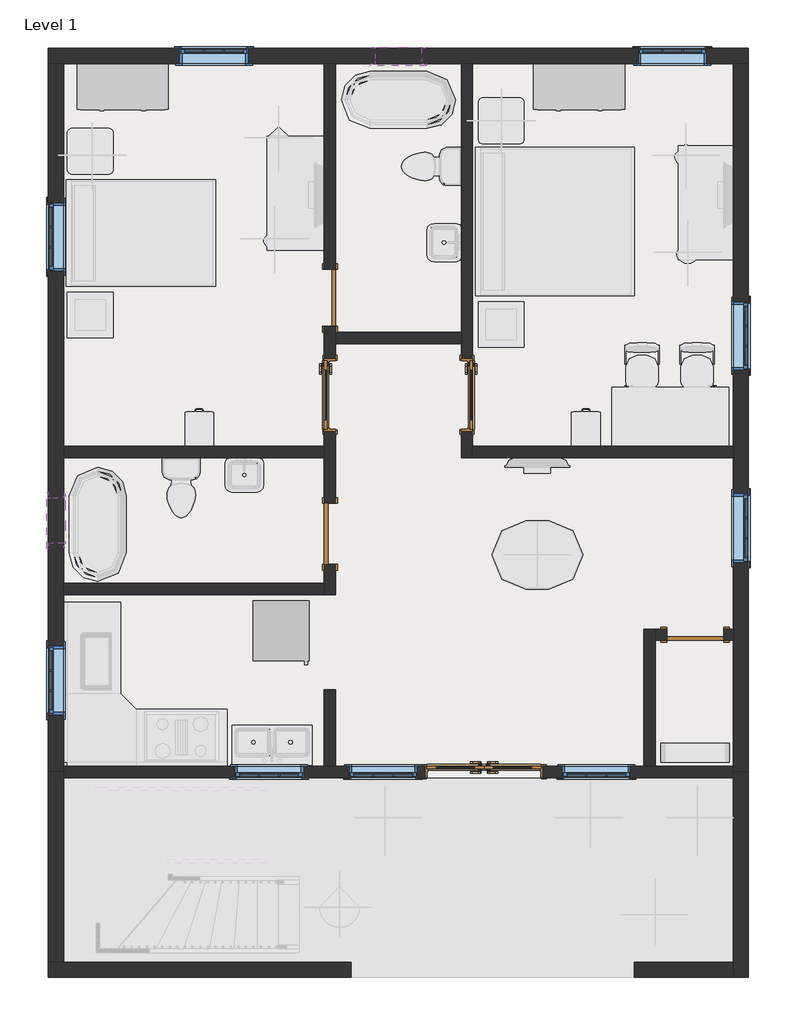
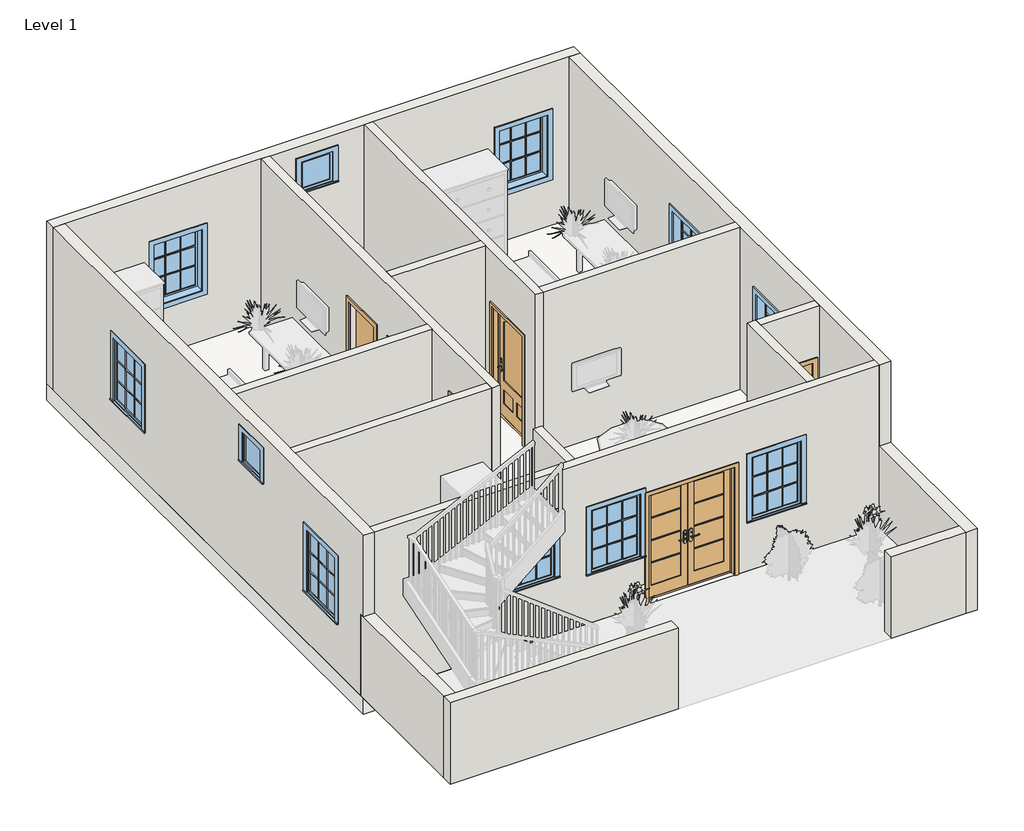
# One storey, part 1 of 3: 17 walls, 11 windows, 6 doors, 1 slab.
"""IFC4 building model written with IfcOpenShell, lengths in millimetres."""

from ifc_helpers import new_model, si_unit, frame, origin, origin_with_axes, place, context, project, spatial, polyline, outline, extrude, faceted_brep, transform, mapped, element, save
from components import door_808aeb8e, door_5d363d20, door_94998e6c, door_059fdd7e, door_bb092f7c, window_29c06734, window_5c190c7e, window_e41d21a6

model = new_model("IFC4")

# Units and contexts
model_context = context("Model", 3, world=origin())
ifc_project = project(units=[si_unit("LENGTHUNIT", "METRE", prefix="MILLI")], contexts=[model_context])

# Site, building, storey
site = spatial("IfcSite", under=ifc_project)
building = spatial("IfcBuilding", under=site)
storey = spatial("IfcBuildingStorey", under=building, Name="Level 1", Elevation=0.0)

# Doors
placement = place(None, origin())
door_shape = door_808aeb8e(model_context)
element("IfcDoor", 1, ObjectType="36\" x 80\"", at=placement, inside=storey, context=model_context, shape_type="MappedRepresentation", body=[
    mapped(door_shape, transform((-7676.9823372, 9599.5174997, 0.0), x_axis=(0.0, 1.0, 0.0), y_axis=(-1.0, 0.0, 0.0), z_axis=(0.0, 0.0, 1.0))),
])
door_2_shape = door_5d363d20(model_context)
element("IfcDoor", 2, ObjectType="36\" x 80\"", at=placement, inside=storey, context=model_context, shape_type="MappedRepresentation", body=[
    mapped(door_2_shape, transform((-5841.8323372, 9599.5174997, 0.0), x_axis=(0.0, 1.0, 0.0), y_axis=(-1.0, 0.0, 0.0), z_axis=(0.0, 0.0, 1.0))),
])
door_3_shape = door_94998e6c(model_context)
element("IfcDoor", 3, ObjectType="Door-Exterior-Double-Full Glass-Wood_Clad : 60\" x 80\"", at=placement, inside=storey, context=model_context, shape_type="MappedRepresentation", body=[
    mapped(door_3_shape, transform((-5616.4073372, 4573.4924997, 0.0), x_axis=(1.0, 0.0, 0.0), y_axis=(0.0, 1.0, 0.0), z_axis=(0.0, 0.0, 1.0))),
])
door_4_shape = door_059fdd7e(model_context)
element("IfcDoor", 4, ObjectType="Single-Flush : 30\" x 80\"", at=placement, inside=storey, context=model_context, shape_type="MappedRepresentation", body=[
    mapped(door_4_shape, transform((-2797.0073372, 6399.1174997, 0.0), x_axis=(-1.0, 0.0, 0.0), y_axis=(0.0, -1.0, 0.0), z_axis=(0.0, 0.0, 1.0))),
])
element("IfcDoor", 5, ObjectType="Single-Flush : 30\" x 80\"", at=placement, inside=storey, context=model_context, shape_type="MappedRepresentation", body=[
    mapped(door_4_shape, transform((-7673.8073372, 10894.9174997, 0.0), x_axis=(0.0, -1.0, 0.0), y_axis=(1.0, 0.0, 0.0), z_axis=(0.0, 0.0, 1.0))),
])
door_5_shape = door_bb092f7c(model_context)
element("IfcDoor", 6, ObjectType="Single-Flush : 32\" x 84\"", at=placement, inside=storey, context=model_context, shape_type="MappedRepresentation", body=[
    mapped(door_5_shape, transform((-7673.8073372, 7745.3174997, 0.0), x_axis=(0.0, -1.0, 0.0), y_axis=(1.0, 0.0, 0.0), z_axis=(0.0, 0.0, 1.0))),
])

# Slab
element("IfcSlab", 7, ObjectType="Generic - 12\"", at=placement, inside=storey, context=model_context, shape_type="SweptSolid", body=[
    extrude(outline(polyline([(-2085.8073372, 14222.3174997), (-2085.8073372, 4494.1174997), (-11433.0073372, 4494.1174997), (-11433.0073372, 14222.3174997), (-2085.8073372, 14222.3174997)])), frame((0.0, 0.0, -304.8), z_axis=(0.0, 0.0, 1.0), x_axis=(1.0, 0.0, 0.0)), (0.0, 0.0, 1.0), 304.8),
])

# Walls
element("IfcWall", 8, ObjectType="Generic - 5'", at=placement, inside=storey, context=model_context, shape_type="SweptSolid", body=[
    extrude(outline(polyline([(-3609.8073372, 2030.3174997), (-2289.0073372, 2030.3174997), (-2289.0073372, 1827.1174997), (-3609.8073372, 1827.1174997), (-3609.8073372, 2030.3174997)])), origin_with_axes(), (0.0, 0.0, 1.0), 1524.0),
])
element("IfcWall", 9, ObjectType="Generic - 5'", at=placement, inside=storey, context=model_context, shape_type="Brep", body=[
    faceted_brep([(-11229.8073372, 2030.3174997, 0.0), (-11229.8073372, 4494.1174997, 0.0), (-11229.8073372, 4570.3174997, 0.0), (-11229.8073372, 4570.3174997, 1524.0), (-11229.8073372, 2030.3174997, 1524.0), (-11433.0073372, 2030.3174997, 0.0), (-11433.0073372, 2030.3174997, 1524.0), (-11433.0073372, 4570.3174997, 1524.0), (-11433.0073372, 4570.3174997, 0.0)], [[[0, 1, 2, 3, 4]], [[5, 6, 7, 8]], [[2, 1, 0, 5, 8]], [[3, 2, 8, 7]], [[4, 3, 7, 6]], [[0, 4, 6, 5]]]),
])
element("IfcWall", 10, ObjectType="Generic - 5'", at=placement, inside=storey, context=model_context, shape_type="Brep", body=[
    faceted_brep([(-2289.0073372, 4570.3174997, 0.0), (-2289.0073372, 4494.1174997, 0.0), (-2289.0073372, 2030.3174997, 0.0), (-2289.0073372, 1827.1174997, 0.0), (-2289.0073372, 1827.1174997, 1524.0), (-2289.0073372, 2030.3174997, 1524.0), (-2289.0073372, 4570.3174997, 1524.0), (-2085.8073372, 4570.3174997, 0.0), (-2085.8073372, 4570.3174997, 1524.0), (-2085.8073372, 1827.1174997, 1524.0), (-2085.8073372, 1827.1174997, 0.0)], [[[0, 1, 2, 3, 4, 5, 6]], [[7, 8, 9, 10]], [[3, 2, 1, 0, 7, 10]], [[6, 5, 4, 9, 8]], [[0, 6, 8, 7]], [[4, 3, 10, 9]]]),
])
element("IfcWall", 11, ObjectType="Generic - 5'", at=placement, inside=storey, context=model_context, shape_type="Brep", body=[
    faceted_brep([(-7394.4073372, 2030.3174997, 0.0), (-11229.8073372, 2030.3174997, 0.0), (-11433.0073372, 2030.3174997, 0.0), (-11433.0073372, 2030.3174997, 1524.0), (-11229.8073372, 2030.3174997, 1524.0), (-7394.4073372, 2030.3174997, 1524.0), (-7394.4073372, 1827.1174997, 0.0), (-7394.4073372, 1827.1174997, 1524.0), (-11433.0073372, 1827.1174997, 1524.0), (-11433.0073372, 1827.1174997, 0.0)], [[[0, 1, 2, 3, 4, 5]], [[6, 7, 8, 9]], [[2, 1, 0, 6, 9]], [[5, 4, 3, 8, 7]], [[0, 5, 7, 6]], [[3, 2, 9, 8]]]),
])
element("IfcWall", 12, ObjectType="Generic - 8\"", at=placement, inside=storey, context=model_context, shape_type="Brep", body=[
    faceted_brep([(-11433.0073372, 14019.1174997, 0.0), (-11229.8073372, 14019.1174997, 0.0), (-7750.0073372, 14019.1174997, 0.0), (-7597.6073372, 14019.1174997, 0.0), (-5921.2073372, 14019.1174997, 0.0), (-5768.8073372, 14019.1174997, 0.0), (-2289.0073372, 14019.1174997, 0.0), (-2085.8073372, 14019.1174997, 0.0), (-2085.8073372, 14019.1174997, 3048.0), (-2289.0073372, 14019.1174997, 3048.0), (-5768.8073372, 14019.1174997, 3048.0), (-5921.2073372, 14019.1174997, 3048.0), (-7597.6073372, 14019.1174997, 3048.0), (-7750.0073372, 14019.1174997, 3048.0), (-11229.8073372, 14019.1174997, 3048.0), (-11433.0073372, 14019.1174997, 3048.0), (-8766.0073372, 14019.1174997, 2133.6), (-8766.0073372, 14019.1174997, 914.4), (-9680.4073372, 14019.1174997, 914.4), (-9680.4073372, 14019.1174997, 2133.6), (-2644.6073372, 14019.1174997, 2133.6), (-2644.6073372, 14019.1174997, 914.4), (-3559.0073372, 14019.1174997, 914.4), (-3559.0073372, 14019.1174997, 2133.6), (-7064.2073372, 14019.1174997, 2768.6), (-6454.6073372, 14019.1174997, 2768.6), (-6454.6073372, 14019.1174997, 2159.0), (-7064.2073372, 14019.1174997, 2159.0), (-11433.0073372, 14222.3174997, 0.0), (-11433.0073372, 14222.3174997, 3048.0), (-2085.8073372, 14222.3174997, 3048.0), (-2085.8073372, 14222.3174997, 0.0), (-8766.0073372, 14222.3174997, 2133.6), (-9680.4073372, 14222.3174997, 2133.6), (-9680.4073372, 14222.3174997, 914.4), (-8766.0073372, 14222.3174997, 914.4), (-2644.6073372, 14222.3174997, 2133.6), (-3559.0073372, 14222.3174997, 2133.6), (-3559.0073372, 14222.3174997, 914.4), (-2644.6073372, 14222.3174997, 914.4), (-7064.2073372, 14222.3174997, 2768.6), (-7064.2073372, 14222.3174997, 2159.0), (-6454.6073372, 14222.3174997, 2159.0), (-6454.6073372, 14222.3174997, 2768.6)], [[[0, 1, 2, 3, 4, 5, 6, 7, 8, 9, 10, 11, 12, 13, 14, 15], [16, 17, 18, 19], [20, 21, 22, 23], [24, 25, 26, 27]], [[28, 29, 30, 31], [32, 33, 34, 35], [36, 37, 38, 39], [40, 41, 42, 43]], [[7, 6, 5, 4, 3, 2, 1, 0, 28, 31]], [[8, 7, 31, 30]], [[0, 15, 29, 28]], [[17, 16, 32, 35]], [[18, 17, 35, 34]], [[19, 18, 34, 33]], [[16, 19, 33, 32]], [[21, 20, 36, 39]], [[22, 21, 39, 38]], [[23, 22, 38, 37]], [[20, 23, 37, 36]], [[41, 40, 24, 27]], [[42, 41, 27, 26]], [[43, 42, 26, 25]], [[40, 43, 25, 24]], [[15, 14, 13, 12, 11, 10, 9, 8, 30, 29]]]),
])
element("IfcWall", 13, ObjectType="Generic - 8\"", at=placement, inside=storey, context=model_context, shape_type="Brep", body=[
    faceted_brep([(-2289.0073372, 14019.1174997, 0.0), (-2289.0073372, 8913.7174997, 0.0), (-2289.0073372, 8761.3174997, 0.0), (-2289.0073372, 6475.3174997, 0.0), (-2289.0073372, 6322.9174997, 0.0), (-2289.0073372, 4646.5174997, 0.0), (-2289.0073372, 4570.3174997, 0.0), (-2289.0073372, 4570.3174997, 1524.0), (-2289.0073372, 4494.1174997, 1524.0), (-2289.0073372, 4494.1174997, 3048.0), (-2289.0073372, 4646.5174997, 3048.0), (-2289.0073372, 6322.9174997, 3048.0), (-2289.0073372, 6475.3174997, 3048.0), (-2289.0073372, 8761.3174997, 3048.0), (-2289.0073372, 8913.7174997, 3048.0), (-2289.0073372, 14019.1174997, 3048.0), (-2289.0073372, 7364.3174997, 2133.6), (-2289.0073372, 7364.3174997, 914.4), (-2289.0073372, 8278.7174997, 914.4), (-2289.0073372, 8278.7174997, 2133.6), (-2289.0073372, 9929.7174997, 2133.6), (-2289.0073372, 9929.7174997, 914.4), (-2289.0073372, 10844.1174997, 914.4), (-2289.0073372, 10844.1174997, 2133.6), (-2085.8073372, 14019.1174997, 0.0), (-2085.8073372, 14019.1174997, 3048.0), (-2085.8073372, 4494.1174997, 3048.0), (-2085.8073372, 4494.1174997, 1524.0), (-2085.8073372, 4570.3174997, 1524.0), (-2085.8073372, 4570.3174997, 0.0), (-2085.8073372, 7364.3174997, 2133.6), (-2085.8073372, 8278.7174997, 2133.6), (-2085.8073372, 8278.7174997, 914.4), (-2085.8073372, 7364.3174997, 914.4), (-2085.8073372, 9929.7174997, 2133.6), (-2085.8073372, 10844.1174997, 2133.6), (-2085.8073372, 10844.1174997, 914.4), (-2085.8073372, 9929.7174997, 914.4)], [[[0, 1, 2, 3, 4, 5, 6, 7, 8, 9, 10, 11, 12, 13, 14, 15], [16, 17, 18, 19], [20, 21, 22, 23]], [[24, 25, 26, 27, 28, 29], [30, 31, 32, 33], [34, 35, 36, 37]], [[6, 5, 4, 3, 2, 1, 0, 24, 29]], [[0, 15, 25, 24]], [[17, 16, 30, 33]], [[18, 17, 33, 32]], [[19, 18, 32, 31]], [[16, 19, 31, 30]], [[21, 20, 34, 37]], [[22, 21, 37, 36]], [[23, 22, 36, 35]], [[20, 23, 35, 34]], [[7, 6, 29, 28]], [[27, 8, 7, 28]], [[9, 8, 27, 26]], [[15, 14, 13, 12, 11, 10, 9, 26, 25]]]),
])
element("IfcWall", 14, ObjectType="Generic - 8\"", at=placement, inside=storey, context=model_context, shape_type="Brep", body=[
    faceted_brep([(-11229.8073372, 4570.3174997, 0.0), (-11229.8073372, 4646.5174997, 0.0), (-11229.8073372, 6932.5174997, 0.0), (-11229.8073372, 7084.9174997, 0.0), (-11229.8073372, 8761.3174997, 0.0), (-11229.8073372, 8913.7174997, 0.0), (-11229.8073372, 14019.1174997, 0.0), (-11229.8073372, 14019.1174997, 3048.0), (-11229.8073372, 8913.7174997, 3048.0), (-11229.8073372, 8761.3174997, 3048.0), (-11229.8073372, 7084.9174997, 3048.0), (-11229.8073372, 6932.5174997, 3048.0), (-11229.8073372, 4646.5174997, 3048.0), (-11229.8073372, 4494.1174997, 3048.0), (-11229.8073372, 4494.1174997, 1524.0), (-11229.8073372, 4570.3174997, 1524.0), (-11229.8073372, 12164.9174997, 2133.6), (-11229.8073372, 12164.9174997, 914.4), (-11229.8073372, 11250.5174997, 914.4), (-11229.8073372, 11250.5174997, 2133.6), (-11229.8073372, 6246.7174997, 2133.6), (-11229.8073372, 6246.7174997, 914.4), (-11229.8073372, 5332.3174997, 914.4), (-11229.8073372, 5332.3174997, 2133.6), (-11229.8073372, 8227.9174997, 2768.6), (-11229.8073372, 8227.9174997, 2159.0), (-11229.8073372, 7618.3174997, 2159.0), (-11229.8073372, 7618.3174997, 2768.6), (-11433.0073372, 4570.3174997, 0.0), (-11433.0073372, 4570.3174997, 1524.0), (-11433.0073372, 4494.1174997, 1524.0), (-11433.0073372, 4494.1174997, 3048.0), (-11433.0073372, 14019.1174997, 3048.0), (-11433.0073372, 14019.1174997, 0.0), (-11433.0073372, 12164.9174997, 2133.6), (-11433.0073372, 11250.5174997, 2133.6), (-11433.0073372, 11250.5174997, 914.4), (-11433.0073372, 12164.9174997, 914.4), (-11433.0073372, 6246.7174997, 2133.6), (-11433.0073372, 5332.3174997, 2133.6), (-11433.0073372, 5332.3174997, 914.4), (-11433.0073372, 6246.7174997, 914.4), (-11433.0073372, 8227.9174997, 2768.6), (-11433.0073372, 7618.3174997, 2768.6), (-11433.0073372, 7618.3174997, 2159.0), (-11433.0073372, 8227.9174997, 2159.0)], [[[0, 1, 2, 3, 4, 5, 6, 7, 8, 9, 10, 11, 12, 13, 14, 15], [16, 17, 18, 19], [20, 21, 22, 23], [24, 25, 26, 27]], [[28, 29, 30, 31, 32, 33], [34, 35, 36, 37], [38, 39, 40, 41], [42, 43, 44, 45]], [[6, 5, 4, 3, 2, 1, 0, 28, 33]], [[7, 6, 33, 32]], [[17, 16, 34, 37]], [[18, 17, 37, 36]], [[19, 18, 36, 35]], [[16, 19, 35, 34]], [[21, 20, 38, 41]], [[22, 21, 41, 40]], [[23, 22, 40, 39]], [[20, 23, 39, 38]], [[25, 24, 42, 45]], [[26, 25, 45, 44]], [[27, 26, 44, 43]], [[24, 27, 43, 42]], [[0, 15, 29, 28]], [[14, 30, 29, 15]], [[14, 13, 31, 30]], [[13, 12, 11, 10, 9, 8, 7, 32, 31]]]),
])
element("IfcWall", 15, ObjectType="INNER 6\"", at=placement, inside=storey, context=model_context, shape_type="Brep", body=[
    faceted_brep([(-7750.0073372, 10513.9174997, 2032.0), (-7750.0073372, 10513.9174997, 0.0), (-7750.0073372, 10082.1174997, 0.0), (-7750.0073372, 10082.1174997, 2057.4), (-7750.0073372, 9116.9174997, 2057.4), (-7750.0073372, 9116.9174997, 0.0), (-7750.0073372, 8913.7174997, 0.0), (-7750.0073372, 8761.3174997, 0.0), (-7750.0073372, 8151.7174997, 0.0), (-7750.0073372, 8151.7174997, 2133.6), (-7750.0073372, 7338.9174997, 2133.6), (-7750.0073372, 7338.9174997, 0.0), (-7750.0073372, 7084.9174997, 0.0), (-7750.0073372, 6932.5174997, 0.0), (-7750.0073372, 6932.5174997, 3048.0), (-7750.0073372, 7084.9174997, 3048.0), (-7750.0073372, 8761.3174997, 3048.0), (-7750.0073372, 8913.7174997, 3048.0), (-7750.0073372, 14019.1174997, 3048.0), (-7750.0073372, 14019.1174997, 0.0), (-7750.0073372, 11275.9174997, 0.0), (-7750.0073372, 11275.9174997, 2032.0), (-7597.6073372, 10082.1174997, 0.0), (-7597.6073372, 10285.3174997, 0.0), (-7597.6073372, 10437.7174997, 0.0), (-7597.6073372, 10513.9174997, 0.0), (-7597.6073372, 10513.9174997, 2032.0), (-7597.6073372, 11275.9174997, 2032.0), (-7597.6073372, 11275.9174997, 0.0), (-7597.6073372, 14019.1174997, 0.0), (-7597.6073372, 14019.1174997, 3048.0), (-7597.6073372, 10437.7174997, 3048.0), (-7597.6073372, 10285.3174997, 3048.0), (-7597.6073372, 6932.5174997, 3048.0), (-7597.6073372, 6932.5174997, 0.0), (-7597.6073372, 7338.9174997, 0.0), (-7597.6073372, 7338.9174997, 2133.6), (-7597.6073372, 8151.7174997, 2133.6), (-7597.6073372, 8151.7174997, 0.0), (-7597.6073372, 9116.9174997, 0.0), (-7597.6073372, 9116.9174997, 2057.4), (-7597.6073372, 10082.1174997, 2057.4)], [[[0, 1, 2, 3, 4, 5, 6, 7, 8, 9, 10, 11, 12, 13, 14, 15, 16, 17, 18, 19, 20, 21]], [[22, 23, 24, 25, 26, 27, 28, 29, 30, 31, 32, 33, 34, 35, 36, 37, 38, 39, 40, 41]], [[11, 35, 34, 13, 12]], [[38, 8, 7, 6, 5, 39]], [[20, 19, 29, 28]], [[2, 1, 25, 24, 23, 22]], [[19, 18, 30, 29]], [[36, 35, 11, 10]], [[37, 36, 10, 9]], [[38, 37, 9, 8]], [[41, 3, 2, 22]], [[3, 41, 40, 4]], [[4, 40, 39, 5]], [[14, 13, 34, 33]], [[26, 25, 1, 0]], [[27, 26, 0, 21]], [[28, 27, 21, 20]], [[18, 17, 16, 15, 14, 33, 32, 31, 30]]]),
])
element("IfcWall", 16, ObjectType="INNER 6\"", at=placement, inside=storey, context=model_context, shape_type="SweptSolid", body=[
    extrude(outline(polyline([(-11229.8073372, 8913.7174997), (-7750.0073372, 8913.7174997), (-7750.0073372, 8761.3174997), (-11229.8073372, 8761.3174997), (-11229.8073372, 8913.7174997)])), origin_with_axes(), (0.0, 0.0, 1.0), 3048.0),
])
element("IfcWall", 17, ObjectType="INNER 6\"", at=placement, inside=storey, context=model_context, shape_type="Brep", body=[
    faceted_brep([(-5921.2073372, 14019.1174997, 3048.0), (-5921.2073372, 14019.1174997, 0.0), (-5921.2073372, 10437.7174997, 0.0), (-5921.2073372, 10285.3174997, 0.0), (-5921.2073372, 10082.1174997, 0.0), (-5921.2073372, 10082.1174997, 2057.4), (-5921.2073372, 9116.9174997, 2057.4), (-5921.2073372, 9116.9174997, 0.0), (-5921.2073372, 8761.3174997, 0.0), (-5921.2073372, 8761.3174997, 3048.0), (-5921.2073372, 10285.3174997, 3048.0), (-5921.2073372, 10437.7174997, 3048.0), (-5768.8073372, 14019.1174997, 0.0), (-5768.8073372, 14019.1174997, 3048.0), (-5768.8073372, 8913.7174997, 3048.0), (-5768.8073372, 8761.3174997, 3048.0), (-5768.8073372, 8761.3174997, 0.0), (-5768.8073372, 8913.7174997, 0.0), (-5768.8073372, 9116.9174997, 0.0), (-5768.8073372, 9116.9174997, 2057.4), (-5768.8073372, 10082.1174997, 2057.4), (-5768.8073372, 10082.1174997, 0.0)], [[[0, 1, 2, 3, 4, 5, 6, 7, 8, 9, 10, 11]], [[12, 13, 14, 15, 16, 17, 18, 19, 20, 21]], [[1, 12, 21, 4, 3, 2]], [[16, 8, 7, 18, 17]], [[1, 0, 13, 12]], [[9, 8, 16, 15]], [[20, 5, 4, 21]], [[5, 20, 19, 6]], [[6, 19, 18, 7]], [[0, 11, 10, 9, 15, 14, 13]]]),
])
element("IfcWall", 18, ObjectType="INNER 6\"", at=placement, inside=storey, context=model_context, shape_type="SweptSolid", body=[
    extrude(outline(polyline([(-7597.6073372, 10437.7174997), (-5921.2073372, 10437.7174997), (-5921.2073372, 10285.3174997), (-7597.6073372, 10285.3174997), (-7597.6073372, 10437.7174997)])), origin_with_axes(), (0.0, 0.0, 1.0), 3048.0),
])
element("IfcWall", 19, ObjectType="INNER 6\"", at=placement, inside=storey, context=model_context, shape_type="SweptSolid", body=[
    extrude(outline(polyline([(-2289.0073372, 8761.3174997), (-5768.8073372, 8761.3174997), (-5768.8073372, 8913.7174997), (-2289.0073372, 8913.7174997), (-2289.0073372, 8761.3174997)])), origin_with_axes(), (0.0, 0.0, 1.0), 3048.0),
])
element("IfcWall", 20, ObjectType="INNER 6\"", at=placement, inside=storey, context=model_context, shape_type="SweptSolid", body=[
    extrude(outline(polyline([(-7750.0073372, 6932.5174997), (-11229.8073372, 6932.5174997), (-11229.8073372, 7084.9174997), (-7750.0073372, 7084.9174997), (-7750.0073372, 6932.5174997)])), origin_with_axes(), (0.0, 0.0, 1.0), 3048.0),
])
element("IfcWall", 21, ObjectType="INNER 6\"", at=placement, inside=storey, context=model_context, shape_type="Brep", body=[
    faceted_brep([(-2289.0073372, 4494.1174997, 0.0), (-2289.0073372, 4494.1174997, 1524.0), (-2289.0073372, 4494.1174997, 3048.0), (-11229.8073372, 4494.1174997, 3048.0), (-11229.8073372, 4494.1174997, 1524.0), (-11229.8073372, 4494.1174997, 0.0), (-6403.8073372, 4494.1174997, 0.0), (-6403.8073372, 4494.1174997, 2057.4), (-4829.0073372, 4494.1174997, 2057.4), (-4829.0073372, 4494.1174997, 0.0), (-8943.8073372, 4494.1174997, 2286.0), (-8029.4073372, 4494.1174997, 2286.0), (-8029.4073372, 4494.1174997, 1066.8), (-8943.8073372, 4494.1174997, 1066.8), (-7419.8073372, 4494.1174997, 2133.6), (-6505.4073372, 4494.1174997, 2133.6), (-6505.4073372, 4494.1174997, 914.4), (-7419.8073372, 4494.1174997, 914.4), (-4575.0073372, 4494.1174997, 2133.6), (-3660.6073372, 4494.1174997, 2133.6), (-3660.6073372, 4494.1174997, 914.4), (-4575.0073372, 4494.1174997, 914.4), (-2289.0073372, 4646.5174997, 3048.0), (-2289.0073372, 4646.5174997, 0.0), (-3330.4073372, 4646.5174997, 0.0), (-3482.8073372, 4646.5174997, 0.0), (-4829.0073372, 4646.5174997, 0.0), (-4829.0073372, 4646.5174997, 2057.4), (-6403.8073372, 4646.5174997, 2057.4), (-6403.8073372, 4646.5174997, 0.0), (-7597.6073372, 4646.5174997, 0.0), (-7750.0073372, 4646.5174997, 0.0), (-11229.8073372, 4646.5174997, 0.0), (-11229.8073372, 4646.5174997, 3048.0), (-7750.0073372, 4646.5174997, 3048.0), (-7597.6073372, 4646.5174997, 3048.0), (-3482.8073372, 4646.5174997, 3048.0), (-3330.4073372, 4646.5174997, 3048.0), (-8943.8073372, 4646.5174997, 2286.0), (-8943.8073372, 4646.5174997, 1066.8), (-8029.4073372, 4646.5174997, 1066.8), (-8029.4073372, 4646.5174997, 2286.0), (-7419.8073372, 4646.5174997, 2133.6), (-7419.8073372, 4646.5174997, 914.4), (-6505.4073372, 4646.5174997, 914.4), (-6505.4073372, 4646.5174997, 2133.6), (-4575.0073372, 4646.5174997, 2133.6), (-4575.0073372, 4646.5174997, 914.4), (-3660.6073372, 4646.5174997, 914.4), (-3660.6073372, 4646.5174997, 2133.6), (-2289.0073372, 4570.3174997, 0.0), (-11229.8073372, 4570.3174997, 0.0)], [[[0, 1, 2, 3, 4, 5, 6, 7, 8, 9], [10, 11, 12, 13], [14, 15, 16, 17], [18, 19, 20, 21]], [[22, 23, 24, 25, 26, 27, 28, 29, 30, 31, 32, 33, 34, 35, 36, 37], [38, 39, 40, 41], [42, 43, 44, 45], [46, 47, 48, 49]], [[23, 50, 0, 9, 26, 25, 24]], [[5, 51, 32, 31, 30, 29, 6]], [[8, 27, 26, 9]], [[27, 8, 7, 28]], [[28, 7, 6, 29]], [[39, 38, 10, 13]], [[40, 39, 13, 12]], [[41, 40, 12, 11]], [[38, 41, 11, 10]], [[43, 42, 14, 17]], [[44, 43, 17, 16]], [[45, 44, 16, 15]], [[42, 45, 15, 14]], [[47, 46, 18, 21]], [[48, 47, 21, 20]], [[49, 48, 20, 19]], [[46, 49, 19, 18]], [[0, 50, 23, 22, 2, 1]], [[32, 51, 5, 4, 3, 33]], [[3, 2, 22, 37, 36, 35, 34, 33]]]),
])
element("IfcWall", 22, ObjectType="INNER 6\"", at=placement, inside=storey, context=model_context, shape_type="Brep", body=[
    faceted_brep([(-3330.4073372, 4646.5174997, 0.0), (-3330.4073372, 6322.9174997, 0.0), (-3330.4073372, 6475.3174997, 0.0), (-3330.4073372, 6475.3174997, 3048.0), (-3330.4073372, 6322.9174997, 3048.0), (-3330.4073372, 4646.5174997, 3048.0), (-3482.8073372, 4646.5174997, 0.0), (-3482.8073372, 4646.5174997, 3048.0), (-3482.8073372, 6475.3174997, 3048.0), (-3482.8073372, 6475.3174997, 0.0)], [[[0, 1, 2, 3, 4, 5]], [[6, 7, 8, 9]], [[2, 1, 0, 6, 9]], [[0, 5, 7, 6]], [[3, 2, 9, 8]], [[5, 4, 3, 8, 7]]]),
])
element("IfcWall", 23, ObjectType="INNER 6\"", at=placement, inside=storey, context=model_context, shape_type="SweptSolid", body=[
    extrude(outline(polyline([(0.0, -3330.4073372), (0.0, -3178.0073372), (2032.0, -3178.0073372), (2032.0, -2416.0073372), (0.0, -2416.0073372), (0.0, -2289.0073372), (3048.0, -2289.0073372), (3048.0, -3330.4073372), (0.0, -3330.4073372)])), frame((0.0, 6322.9174997, 0.0), z_axis=(0.0, 1.0, 0.0), x_axis=(0.0, 0.0, 1.0)), (0.0, 0.0, 1.0), 152.4),
])
element("IfcWall", 24, ObjectType="INNER 6\"", at=placement, inside=storey, context=model_context, shape_type="SweptSolid", body=[
    extrude(outline(polyline([(-7750.0073372, 4646.5174997), (-7750.0073372, 5662.5174997), (-7597.6073372, 5662.5174997), (-7597.6073372, 4646.5174997), (-7750.0073372, 4646.5174997)])), origin_with_axes(), (0.0, 0.0, 1.0), 3048.0),
])

# Windows
window_shape = window_29c06734(model_context)
element("IfcWindow", 25, ObjectType="Casement 3x3 with Trim : 36\" x 48\"", at=placement, inside=storey, context=model_context, shape_type="MappedRepresentation", body=[
    mapped(window_shape, transform((-9223.2073372, 14120.7174997, 0.0), x_axis=(1.0, 0.0, 0.0), y_axis=(0.0, 1.0, 0.0), z_axis=(0.0, 0.0, 1.0))),
])
element("IfcWindow", 26, ObjectType="Casement 3x3 with Trim : 36\" x 48\"", at=placement, inside=storey, context=model_context, shape_type="MappedRepresentation", body=[
    mapped(window_shape, transform((-11331.4073372, 11707.7174997, 0.0), x_axis=(0.0, 1.0, 0.0), y_axis=(-1.0, 0.0, 0.0), z_axis=(0.0, 0.0, 1.0))),
])
element("IfcWindow", 27, ObjectType="Casement 3x3 with Trim : 36\" x 48\"", at=placement, inside=storey, context=model_context, shape_type="MappedRepresentation", body=[
    mapped(window_shape, transform((-11331.4073372, 5789.5174997, 0.0), x_axis=(0.0, 1.0, 0.0), y_axis=(-1.0, 0.0, 0.0), z_axis=(0.0, 0.0, 1.0))),
])
element("IfcWindow", 28, ObjectType="Casement 3x3 with Trim : 36\" x 48\"", at=placement, inside=storey, context=model_context, shape_type="MappedRepresentation", body=[
    mapped(window_shape, transform((-2187.4073372, 7821.5174997, 0.0), x_axis=(0.0, -1.0, 0.0), y_axis=(1.0, 0.0, 0.0), z_axis=(0.0, 0.0, 1.0))),
])
element("IfcWindow", 29, ObjectType="Casement 3x3 with Trim : 36\" x 48\"", at=placement, inside=storey, context=model_context, shape_type="MappedRepresentation", body=[
    mapped(window_shape, transform((-2187.4073372, 10386.9174997, 0.0), x_axis=(0.0, -1.0, 0.0), y_axis=(1.0, 0.0, 0.0), z_axis=(0.0, 0.0, 1.0))),
])
element("IfcWindow", 30, ObjectType="Casement 3x3 with Trim : 36\" x 48\"", at=placement, inside=storey, context=model_context, shape_type="MappedRepresentation", body=[
    mapped(window_shape, transform((-3101.8073372, 14120.7174997, 0.0), x_axis=(1.0, 0.0, 0.0), y_axis=(0.0, 1.0, 0.0), z_axis=(0.0, 0.0, 1.0))),
])
window_2_shape = window_5c190c7e(model_context)
element("IfcWindow", 31, ObjectType="Casement 3x3 with Trim : 36\" x 48\"", at=placement, inside=storey, context=model_context, shape_type="MappedRepresentation", body=[
    mapped(window_2_shape, transform((-8486.6073372, 4570.3174997, 152.4), x_axis=(-1.0, 0.0, 0.0), y_axis=(0.0, -1.0, 0.0), z_axis=(0.0, 0.0, 1.0))),
])
element("IfcWindow", 32, ObjectType="Casement 3x3 with Trim : 36\" x 48\"", at=placement, inside=storey, context=model_context, shape_type="MappedRepresentation", body=[
    mapped(window_2_shape, transform((-6962.6073372, 4570.3174997, 0.0), x_axis=(-1.0, 0.0, 0.0), y_axis=(0.0, -1.0, 0.0), z_axis=(0.0, 0.0, 1.0))),
])
element("IfcWindow", 33, ObjectType="Casement 3x3 with Trim : 36\" x 48\"", at=placement, inside=storey, context=model_context, shape_type="MappedRepresentation", body=[
    mapped(window_2_shape, transform((-4117.8073372, 4570.3174997, 0.0), x_axis=(-1.0, 0.0, 0.0), y_axis=(0.0, -1.0, 0.0), z_axis=(0.0, 0.0, 1.0))),
])
window_3_shape = window_e41d21a6(model_context)
element("IfcWindow", 34, ObjectType="Transom with Trim : 24\" x 24\"", at=placement, inside=storey, context=model_context, shape_type="MappedRepresentation", body=[
    mapped(window_3_shape, transform((-6797.5073372, 14120.7174997, 0.0), x_axis=(-1.0, 0.0, 0.0), y_axis=(0.0, -1.0, 0.0), z_axis=(0.0, 0.0, 1.0))),
])
element("IfcWindow", 35, ObjectType="Transom with Trim : 24\" x 24\"", at=placement, inside=storey, context=model_context, shape_type="MappedRepresentation", body=[
    mapped(window_3_shape, transform((-11331.4073372, 7961.2174997, 0.0), x_axis=(0.0, 1.0, 0.0), y_axis=(-1.0, 0.0, 0.0), z_axis=(0.0, 0.0, 1.0))),
])

save(model, "model.ifc")

# Revit data of these elements
# Type "36\" x 80\""
#   Type Mark = "8"
#   Assembly Code = "B2030100"
#   Analytic Construction = "French door, wood frame with single glass"
#   Threshold Offset [instance default] = 0' - 0 1/2"
#   Thickness = 0' - 1 3/8"
#   Thermal Resistance (R) = 1.0696 (h·ft²·°F)/BTU
#   Swing Angle [instance default] = 90.00°
#   Stiles = 0' - 4 3/4"
#   Rough Width = 3' - 2"
#   Rough Height = 6' - 9"
#   Radius = 1' - 8.05625"
#   Lock Rail = 0' - 7 1/8"
#   Height = 6' - 8"
#   Width = 3' - 0"
#   Heat Transfer Coefficient (U) = 0.9350 BTU/(h·ft²·°F)
#   Door Offset [instance default] = 0' - 0"
#   Bottom Rail = 0' - 9 1/2"
#   Threshold [instance default] = yes
#   Function = 1
#   Exterior Trim [instance default] = yes
#   Trim Material = Cherry
#   Threshold Material = Cherry
#   Panel Material = Cherry
#   Glazing = Glass
#   Frame Material = Cherry
#   Door Handle Material = Aluminum
#   Visual Light Transmittance = 0
#   Solar Heat Gain Coefficient = 0
#   Wall Closure = (empty or 0)
#   Construction Type = (empty or 0)
# Type "Door-Exterior-Double-Full Glass-Wood_Clad : 60\" x 80\""
#   Type Mark = "9"
#   Assembly Code = "B2030100"
#   Analytic Construction = "French door, wood frame with double glass"
#   Top Rail = 0' - 4 11/16"
#   Threshold Offset [instance default] = 0' - 0 1/2"
#   Thickness = 0' - 1 3/8"
#   Thermal Resistance (R) = 1.9158 (h·ft²·°F)/BTU
#   Swing Angle [instance default] = 90.00°
#   Stiles = 0' - 4 3/4"
#   Rough Width = 5' - 2"
#   Rough Height = 6' - 9"
#   Panel Width = 2' - 6"
#   Door Offset [instance default] = 0' - 0"
#   Height = 6' - 8"
#   Width = 5' - 0"
#   Heat Transfer Coefficient (U) = 0.5220 BTU/(h·ft²·°F)
#   Bottom Rail = 0' - 9 1/8"
#   Exterior Trim [instance default] = yes
#   Threshold [instance default] = yes
#   Show Grill [instance default] = yes
#   Function = 1
#   Trim Material = Cherry
#   Threshold Material = Cherry
#   Panel Material = Cherry
#   Glazing = Glass
#   Frame Material = Cherry
#   Door Handle Material = Aluminum
#   Visual Light Transmittance = 0
#   Solar Heat Gain Coefficient = 0
#   Wall Closure = (empty or 0)
#   Construction Type = (empty or 0)
# Type "Single-Flush : 30\" x 80\""
#   Type Mark = "5"
#   Construction Type Id = "MDOOR"
#   Assembly Code = "C1020"
#   Analytic Construction = "Metal"
#   Thickness = 0' - 2"
#   Heat Transfer Coefficient (U) = 0.651978 BTU/(h·ft²·°F)
#   Height = 6' - 8"
#   Trim Projection Ext = 0' - 1"
#   Trim Projection Int = 0' - 1"
#   Trim Width = 0' - 3"
#   Width = 2' - 6"
#   Define Thermal Properties by = 1
#   Door Material = Door - Panel
#   Frame Material = Door - Frame
#   Visual Light Transmittance = 0
#   Solar Heat Gain Coefficient = 0
#   Function = (empty or 0)
#   Wall Closure = (empty or 0)
# Type "Single-Flush : 32\" x 84\""
#   Type Mark = "3"
#   Construction Type Id = "MDOOR"
#   Assembly Code = "C1020"
#   Analytic Construction = "Metal"
#   Thickness = 0' - 2"
#   Heat Transfer Coefficient (U) = 0.651978 BTU/(h·ft²·°F)
#   Height = 7' - 0"
#   Trim Projection Ext = 0' - 1"
#   Trim Projection Int = 0' - 1"
#   Trim Width = 0' - 3"
#   Width = 2' - 8"
#   Define Thermal Properties by = 1
#   Door Material = Door - Panel
#   Frame Material = Door - Frame
#   Visual Light Transmittance = 0
#   Solar Heat Gain Coefficient = 0
#   Function = (empty or 0)
#   Wall Closure = (empty or 0)
# Type "Generic - 12\""
#   Assembly Code = "B1010"
#   Function = 0
#   Layers, outside or top first: 1' - 0" no material (function 1)
# Type "Generic - 5'"
#   Assembly Code = "B2010"
#   Layers, outside or top first: 0' - 8" "Birch" (function 1)
# Type "Generic - 8\""
#   Assembly Code = "B2010"
#   Layers, outside or top first: 0' - 8" "Brick, Common" (function 1)
# Type "INNER 6\""
#   Assembly Code = "B2010"
#   Layers, outside or top first: 0' - 6" "Brick, Common" (function 1)
# Type "Casement 3x3 with Trim : 36\" x 48\""
#   Type Mark = "10"
#   Construction Type Id = "GSP4R"
#   Assembly Code = "B2020100"
#   Analytic Construction = "1/8 in Pilkington single glazing"
#   Visual Light Transmittance = 0.9
#   Solar Heat Gain Coefficient = 0.78
#   Heat Transfer Coefficient (U) = 0.6496 BTU/(h·ft²·°F)
#   Height = 4' - 0"
#   Default Sill Height = 3' - 0"
#   Trim Projection - Ext. = 0' - 0 1/2"
#   Trim Projection - Int. = 0' - 0 3/4"
#   Trim Width - Exterior = 0' - 3 1/2"
#   Trim Width - Interior = 0' - 3 1/2"
#   Width = 3' - 0"
#   Window Inset = 0' - 0 3/4"
#   Define Thermal Properties by = 1
#   Glass Pane Material = Glass
#   Sash Material = Sash
#   Trim Exterior Material = Trim
#   Trim Interior Material = Trim
#   Wall Closure = (empty or 0)
# Type "Transom with Trim : 24\" x 24\""
#   Type Mark = "13"
#   Construction Type Id = "GSP4R"
#   Assembly Code = "B2020100"
#   Analytic Construction = "1/8 in Pilkington single glazing"
#   Visual Light Transmittance = 0.9
#   Solar Heat Gain Coefficient = 0.78
#   Heat Transfer Coefficient (U) = 0.6496 BTU/(h·ft²·°F)
#   Height = 2' - 0"
#   Default Sill Height = 7' - 1"
#   Trim Projection - Ext. = 0' - 0 1/2"
#   Trim Projection - Int. = 0' - 0 3/4"
#   Trim Width - Exterior = 0' - 3 1/2"
#   Trim Width - Interior = 0' - 3 1/2"
#   Width = 2' - 0"
#   Window Inset = 0' - 0 3/4"
#   Define Thermal Properties by = 1
#   Glass Pane Material = Glass
#   Sash Material = Sash
#   Trim Exterior Material = Trim
#   Trim Interior Material = Trim
#   Wall Closure = (empty or 0)
# Elements 1, 2 (IfcDoor, "36\" x 80\"")
#   Threshold Offset = 0' - 0 1/2"
#   Swing Angle = 90.00°
#   Door Offset = 0' - 0"
#   Threshold = yes
#   Exterior Trim = yes
#   Phase Created = New Construction
#   Materials on its faces: "Cherry", "Aluminum", "Glass"
# Element 3 (IfcDoor, "Door-Exterior-Double-Full Glass-Wood_Clad : 60\" x 80\"")
#   Threshold Offset = 0' - 0 1/2"
#   Swing Angle = 90.00°
#   Door Offset = 0' - 0"
#   Threshold = yes
#   Show Grill = yes
#   Exterior Trim = yes
#   Phase Created = New Construction
#   Materials on its faces: "Cherry", "Aluminum", "Glass"
# Elements 4, 5 (IfcDoor, "Single-Flush : 30\" x 80\"")
#   Phase Created = New Construction
#   Materials on its faces: "Door - Frame", "Door - Panel"
# Element 6 (IfcDoor, "Single-Flush : 32\" x 84\"")
#   Phase Created = New Construction
#   Materials on its faces: "Door - Frame", "Door - Panel"
# Element 7 (IfcSlab, "Generic - 12\"")
#   Height Offset From Level = 0' - 0"
#   Phase Created = New Construction
#   Materials on its faces: "Default Floor"
# Elements 8, 9, 10, 11 (IfcWall, "Generic - 5'")
#   Top Offset = 0' - 0"
#   Base Offset = 0' - 0"
#   Unconnected Height = 5' - 0"
#   wall height = 5' - 0"
#   Phase Created = New Construction
#   Base Constraint = Level 1
#   Materials on its faces: "Birch"
# Elements 12, 13, 14 (IfcWall, "Generic - 8\"")
#   Top Offset = 0' - 0"
#   Base Offset = 0' - 0"
#   Unconnected Height = 10' - 0"
#   wall height = 10' - 0"
#   Phase Created = New Construction
#   Base Constraint = Level 1
#   Materials on its faces: "Brick, Common"
# Elements 15, 16, 17, 18, 19, 20, 21, 22, 23, 24 (IfcWall, "INNER 6\"")
#   Top Offset = 0' - 0"
#   Base Offset = 0' - 0"
#   Unconnected Height = 10' - 0"
#   wall height = 10' - 0"
#   Phase Created = New Construction
#   Base Constraint = Level 1
#   Materials on its faces: "Brick, Common"
# Element 25 (IfcWindow, "Casement 3x3 with Trim : 36\" x 48\"")
#   Mark = "1"
#   Phase Created = New Construction
#   Materials on its faces: "Sash", "Glass", "Trim"
# Element 26 (IfcWindow, "Casement 3x3 with Trim : 36\" x 48\"")
#   Mark = "2"
#   Phase Created = New Construction
#   Materials on its faces: "Sash", "Glass", "Trim"
# Element 27 (IfcWindow, "Casement 3x3 with Trim : 36\" x 48\"")
#   Mark = "3"
#   Phase Created = New Construction
#   Materials on its faces: "Sash", "Glass", "Trim"
# Element 28 (IfcWindow, "Casement 3x3 with Trim : 36\" x 48\"")
#   Mark = "8"
#   Phase Created = New Construction
#   Materials on its faces: "Sash", "Glass", "Trim"
# Element 29 (IfcWindow, "Casement 3x3 with Trim : 36\" x 48\"")
#   Mark = "9"
#   Phase Created = New Construction
#   Materials on its faces: "Sash", "Glass", "Trim"
# Element 30 (IfcWindow, "Casement 3x3 with Trim : 36\" x 48\"")
#   Mark = "10"
#   Phase Created = New Construction
#   Materials on its faces: "Sash", "Glass", "Trim"
# Element 31 (IfcWindow, "Casement 3x3 with Trim : 36\" x 48\"")
#   Mark = "4"
#   Phase Created = New Construction
#   Materials on its faces: "Sash", "Glass", "Trim"
# Element 32 (IfcWindow, "Casement 3x3 with Trim : 36\" x 48\"")
#   Mark = "6"
#   Phase Created = New Construction
#   Materials on its faces: "Sash", "Glass", "Trim"
# Element 33 (IfcWindow, "Casement 3x3 with Trim : 36\" x 48\"")
#   Mark = "7"
#   Phase Created = New Construction
#   Materials on its faces: "Sash", "Glass", "Trim"
# Element 34 (IfcWindow, "Transom with Trim : 24\" x 24\"")
#   Mark = "11"
#   Phase Created = New Construction
#   Materials on its faces: "Sash", "Trim", "Glass"
# Element 35 (IfcWindow, "Transom with Trim : 24\" x 24\"")
#   Mark = "12"
#   Phase Created = New Construction
#   Materials on its faces: "Sash", "Trim", "Glass"
# Materials
#   "Cherry": class "Wood", colour RGB 226 177 128, transparency 0, Description = "Prunus Serotina", Cost = 0
#   "Glass": class "Glass", colour RGB 0 128 192, transparency 0.75, Description = "Soda Lime Glass", Cost = 0
#   "Aluminum": class "Metal", colour RGB 247 247 247, transparency 0, Description = "Aluminum 6061", Cost = 0
#   "Door - Panel": class "Wood", colour RGB 210 159 95, transparency 0
#   "Door - Frame": colour RGB 118 70 51, transparency 0
#   "Birch": class "Wood", colour RGB 224 178 126, transparency 0, Description = "Betula Alleghaniensis", Cost = 0
#   "Brick, Common": class "Masonry", colour RGB 170 98 104, transparency 0, Description = "Common brick", Cost = 0
#   "Sash": class "Wood", colour RGB 224 178 126, transparency 0
#   "Trim": class "Wood", colour RGB 224 178 126, transparency 0
#   "Default Floor": colour RGB 128 128 128, transparency 0
# Room at (-9541.021, 11742.085) mm, phase "New Construction", upper level "Level 1", upper offset 10' - 0", lower offset 0' - 0"
#   Number = "1"
#   Name = "MASTER BEDROOM"
# Room at (-6871.496, 11898.226) mm, phase "New Construction", upper level "Level 1", upper offset 10' - 0", lower offset 0' - 0"
#   Number = "2"
# Room at (-6769.896, 9382.966) mm, phase "New Construction", upper level "Level 1", upper offset 10' - 0", lower offset 0' - 0"
#   Number = "3"
#   Name = "PASSAGE"
# Room at (-4232.168, 11478.409) mm, phase "New Construction", upper level "Level 1", upper offset 10' - 0", lower offset 0' - 0"
#   Number = "4"
# Room at (-9363.965, 7758.02) mm, phase "New Construction", upper level "Level 1", upper offset 10' - 0", lower offset 0' - 0"
#   Number = "5"
# Room at (-9401.793, 5840.266) mm, phase "New Construction", upper level "Level 1", upper offset 10' - 0", lower offset 0' - 0"
#   Number = "6"
#   Name = "KITCHEN"
# Room at (-3033.553, 7758.02) mm, phase "New Construction", upper level "Level 1", upper offset 10' - 0", lower offset 0' - 0"
#   Number = "7"
#   Name = "FOYER"
# Room at (-2715.277, 5232.26) mm, phase "New Construction", upper level "Level 1", upper offset 10' - 0", lower offset 0' - 0"
#   Number = "8"
# Room at (-5491.015, 6495.864) mm, phase "New Construction", upper level "Level 1", upper offset 10' - 0", lower offset 0' - 0"
#   Number = "9"
